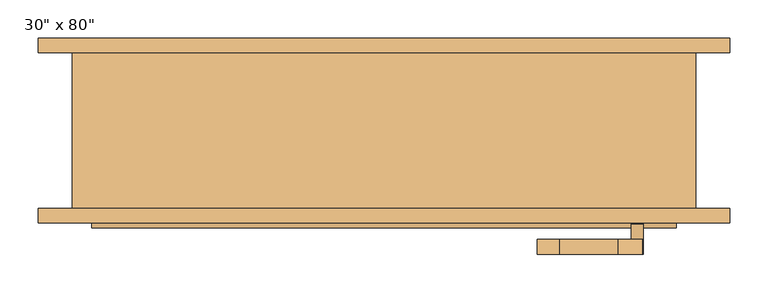
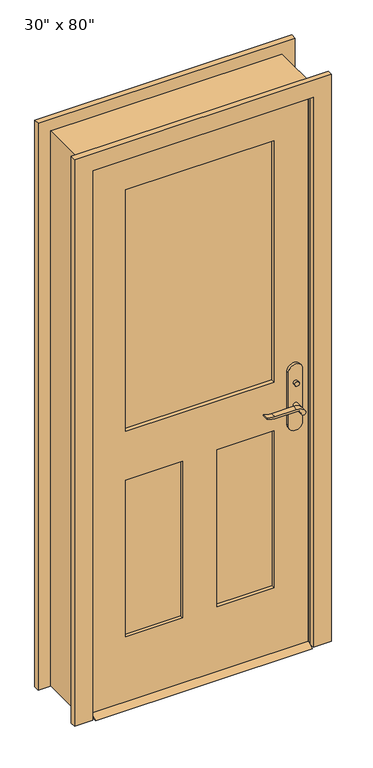
"""IFC4 building model written with IfcOpenShell, lengths in millimetres: door geometry."""

from ifc_helpers import new_model, si_unit, point, frame, frame_2d, origin, place, context, project, spatial, polyline, circle_curve, trimmed, segment, composite_curve, outline, extrude, faceted_brep, source, transform, mapped, element, save


def door_7e6851c9(model_context):
    return source(origin(), model_context, "Body", "SolidModel", [
        extrude(outline(polyline([(-63.5, 12.7), (-38.1, 0.0), (-123.825, 0.0), (-98.425, 12.7), (-63.5, 12.7)])), frame((-381.0, 0.0, 0.0), z_axis=(1.0, 0.0, 0.0), x_axis=(0.0, 1.0, 0.0)), (0.0, 0.0, 1.0), 762.0),
        extrude(outline(polyline([(335.2, -43.5), (335.2, -53.5), (325.2, -53.5), (325.2, -43.5), (335.2, -43.5)])), frame((0.0, 0.0, 981.9), z_axis=(0.0, 0.0, 1.0), x_axis=(1.0, 0.0, 0.0)), (0.0, 0.0, 1.0), 30.0),
        extrude(outline(composite_curve([segment(trimmed(circle_curve(frame_2d((996.9, 330.2)), 8.0), [point((996.9, 322.2))], [point((996.9, 338.2))], False, "CARTESIAN"), True, "CONTINUOUS"), segment(trimmed(circle_curve(frame_2d((996.9, 330.2)), 8.0), [point((996.9, 338.2))], [point((996.9, 322.2))], False, "CARTESIAN"), True, "CONTINUOUS")], self_intersect=False)), frame((0.0, -118.425, 0.0), z_axis=(0.0, 1.0, 0.0), x_axis=(0.0, 0.0, 1.0)), (0.0, 0.0, 1.0), 10.0),
        extrude(outline(composite_curve([segment(trimmed(circle_curve(frame_2d((897.1555521, 306.5324871)), 37.2832219), [point((919.0523287, 336.7081363))], [point((934.4, 304.8325667))], False, "CARTESIAN"), True, "CONTINUOUS"), segment(polyline([(934.4, 304.8325667), (934.4, 228.5564091)]), True, "CONTINUOUS"), segment(trimmed(circle_curve(frame_2d((1017.6850638, 228.6227909)), 83.2850902), [point((934.4, 228.5564091))], [point((939.4, 200.2))], True, "CARTESIAN"), True, "CONTINUOUS"), segment(polyline([(939.4, 200.2), (936.6135558, 200.2)]), True, "CONTINUOUS"), segment(trimmed(circle_curve(frame_2d((986.6709207, 232.1396612)), 59.3791355), [point((936.6135558, 200.2))], [point((927.4, 228.5564091))], False, "CARTESIAN"), True, "CONTINUOUS"), segment(polyline([(927.4, 228.5564091), (927.4, 304.8138099)]), True, "CONTINUOUS"), segment(trimmed(circle_curve(frame_2d((909.2738613, 304.8138099)), 18.1261387), [point((927.4, 304.8138099))], [point((914.4, 322.2))], True, "CARTESIAN"), True, "CONTINUOUS"), segment(trimmed(circle_curve(frame_2d((914.4, 330.2)), 8.0), [point((914.4, 322.2))], [point((919.0523287, 336.7081363))], False, "CARTESIAN"), True, "CONTINUOUS")], self_intersect=False)), frame((0.0, -23.5, 0.0), z_axis=(0.0, 1.0, 0.0), x_axis=(0.0, 0.0, 1.0)), (0.0, 0.0, 1.0), 20.0),
        extrude(outline(composite_curve([segment(trimmed(circle_curve(frame_2d((914.4, 330.2)), 8.0), [point((914.3999903, 322.2))], [point((919.0523287, 336.7081363))], False, "CARTESIAN"), True, "CONTINUOUS"), segment(trimmed(circle_curve(frame_2d((897.1555521, 306.5324871)), 37.2832219), [point((919.0523287, 336.7081363))], [point((934.4, 304.8325667))], False, "CARTESIAN"), True, "CONTINUOUS"), segment(polyline([(934.4, 304.8325667), (934.4, 228.5564091)]), True, "CONTINUOUS"), segment(trimmed(circle_curve(frame_2d((1017.6850638, 228.6227909)), 83.2850902), [point((934.4, 228.5564091))], [point((939.4, 200.2))], True, "CARTESIAN"), True, "CONTINUOUS"), segment(polyline([(939.4, 200.2), (936.6135558, 200.2)]), True, "CONTINUOUS"), segment(trimmed(circle_curve(frame_2d((986.6709207, 232.1396612)), 59.3791355), [point((936.6135558, 200.2))], [point((927.4, 228.5564091))], False, "CARTESIAN"), True, "CONTINUOUS"), segment(polyline([(927.4, 228.5564091), (927.4, 304.8138122)]), True, "CONTINUOUS"), segment(trimmed(circle_curve(frame_2d((909.2738682, 304.8138122)), 18.1261318), [point((927.4, 304.8138122))], [point((914.3999903, 322.2))], True, "CARTESIAN"), True, "CONTINUOUS")], self_intersect=False)), frame((0.0, -158.425, 0.0), z_axis=(0.0, 1.0, 0.0), x_axis=(0.0, 0.0, 1.0)), (0.0, 0.0, 1.0), 20.0),
        extrude(outline(composite_curve([segment(trimmed(circle_curve(frame_2d((914.4, 330.2)), 8.0), [point((914.4, 322.2))], [point((914.4, 338.2))], False, "CARTESIAN"), True, "CONTINUOUS"), segment(trimmed(circle_curve(frame_2d((914.4, 330.2)), 8.0), [point((914.4, 338.2))], [point((914.4, 322.2))], False, "CARTESIAN"), True, "CONTINUOUS")], self_intersect=False)), frame((0.0, -53.5, 0.0), z_axis=(0.0, 1.0, 0.0), x_axis=(0.0, 0.0, 1.0)), (0.0, 0.0, 1.0), 30.0),
        extrude(outline(composite_curve([segment(trimmed(circle_curve(frame_2d((914.4, 330.2)), 8.0), [point((914.4, 322.2))], [point((914.4, 338.2))], False, "CARTESIAN"), True, "CONTINUOUS"), segment(trimmed(circle_curve(frame_2d((914.4, 330.2)), 8.0), [point((914.4, 338.2))], [point((914.4, 322.2))], False, "CARTESIAN"), True, "CONTINUOUS")], self_intersect=False)), frame((0.0, -138.425, 0.0), z_axis=(0.0, 1.0, 0.0), x_axis=(0.0, 0.0, 1.0)), (0.0, 0.0, 1.0), 30.0),
        extrude(outline(composite_curve([segment(polyline([(844.4, 355.2), (1039.4, 355.2)]), True, "CONTINUOUS"), segment(trimmed(circle_curve(frame_2d((1039.4, 330.2)), 25.0), [point((1039.4, 355.2))], [point((1039.4, 305.2))], False, "CARTESIAN"), True, "CONTINUOUS"), segment(polyline([(1039.4, 305.2), (844.4, 305.2)]), True, "CONTINUOUS"), segment(trimmed(circle_curve(frame_2d((844.4, 330.2)), 25.0), [point((844.4, 305.2))], [point((844.4, 355.2))], False, "CARTESIAN"), True, "CONTINUOUS")], self_intersect=False)), frame((0.0, -63.5, 0.0), z_axis=(0.0, 1.0, 0.0), x_axis=(0.0, 0.0, 1.0)), (0.0, 0.0, 1.0), 10.0),
        extrude(outline(composite_curve([segment(polyline([(844.4, 355.2), (1039.4, 355.2)]), True, "CONTINUOUS"), segment(trimmed(circle_curve(frame_2d((1039.4, 330.2)), 25.0), [point((1039.4, 355.2))], [point((1039.4, 305.2))], False, "CARTESIAN"), True, "CONTINUOUS"), segment(polyline([(1039.4, 305.2), (844.4, 305.2)]), True, "CONTINUOUS"), segment(trimmed(circle_curve(frame_2d((844.4, 330.2)), 25.0), [point((844.4, 305.2))], [point((844.4, 355.2))], False, "CARTESIAN"), True, "CONTINUOUS")], self_intersect=False)), frame((0.0, -108.425, 0.0), z_axis=(0.0, 1.0, 0.0), x_axis=(0.0, 0.0, 1.0)), (0.0, 0.0, 1.0), 10.0),
        extrude(outline(polyline([(2032.0, -381.0), (12.7, -381.0), (12.7, 381.0), (2032.0, 381.0), (2032.0, -381.0)]), holes=[polyline([(1016.0, -260.35), (1911.35, -260.35), (1911.35, 260.35), (1016.0, 260.35), (1016.0, -260.35)]), polyline([(835.025, -60.325), (254.0, -60.325), (254.0, -260.35), (835.025, -260.35), (835.025, -60.325)]), polyline([(835.025, 260.35), (254.0, 260.35), (254.0, 60.325), (835.025, 60.325), (835.025, 260.35)])]), frame((0.0, -98.425, 0.0), z_axis=(0.0, 1.0, 0.0), x_axis=(0.0, 0.0, 1.0)), (0.0, 0.0, 1.0), 34.925),
        faceted_brep([(406.4, -98.425, 0.0), (381.0, -98.425, 0.0), (381.0, -63.5, 0.0), (368.3, -63.5, 0.0), (368.3, -28.575, 0.0), (381.0, -28.575, 0.0), (381.0, 104.775, 0.0), (406.4, 104.775, 0.0), (406.4, 104.775, 2057.4), (406.4, -98.425, 2057.4), (381.0, 104.775, 2032.0), (-381.0, 104.775, 2032.0), (-381.0, 104.775, 0.0), (-406.4, 104.775, 0.0), (-406.4, 104.775, 2057.4), (381.0, -28.575, 2032.0), (368.3, -28.575, 2019.3), (-368.3, -28.575, 2019.3), (-368.3, -28.575, 0.0), (-381.0, -28.575, 0.0), (-381.0, -28.575, 2032.0), (368.3, -63.5, 2019.3), (381.0, -63.5, 2032.0), (-381.0, -63.5, 2032.0), (-381.0, -63.5, 0.0), (-368.3, -63.5, 0.0), (-368.3, -63.5, 2019.3), (381.0, -98.425, 2032.0), (-406.4, -98.425, 2057.4), (-406.4, -98.425, 0.0), (-381.0, -98.425, 0.0), (-381.0, -98.425, 2032.0)], [[[0, 1, 2, 3, 4, 5, 6, 7]], [[7, 8, 9, 0]], [[6, 10, 11, 12, 13, 14, 8, 7]], [[5, 15, 10, 6]], [[4, 16, 17, 18, 19, 20, 15, 5]], [[3, 21, 16, 4]], [[2, 22, 23, 24, 25, 26, 21, 3]], [[1, 27, 22, 2]], [[0, 9, 28, 29, 30, 31, 27, 1]], [[8, 14, 28, 9]], [[15, 20, 11, 10]], [[21, 26, 17, 16]], [[27, 31, 23, 22]], [[29, 13, 12, 19, 18, 25, 24, 30]], [[14, 13, 29, 28]], [[20, 19, 12, 11]], [[26, 25, 18, 17]], [[31, 30, 24, 23]]]),
        extrude(outline(polyline([(-60.325, -75.1416667), (-60.325, -86.7833333), (-260.35, -86.7833333), (-260.35, -75.1416667), (-60.325, -75.1416667)])), frame((0.0, 0.0, 254.0), z_axis=(0.0, 0.0, 1.0), x_axis=(1.0, 0.0, 0.0)), (0.0, 0.0, 1.0), 581.025),
        extrude(outline(polyline([(260.35, -75.1416667), (260.35, -86.7833333), (60.325, -86.7833333), (60.325, -75.1416667), (260.35, -75.1416667)])), frame((0.0, 0.0, 254.0), z_axis=(0.0, 0.0, 1.0), x_axis=(1.0, 0.0, 0.0)), (0.0, 0.0, 1.0), 581.025),
        extrude(outline(polyline([(260.35, -77.47), (260.35, -84.455), (-260.35, -84.455), (-260.35, -77.47), (260.35, -77.47)])), frame((0.0, 0.0, 1016.0), z_axis=(0.0, 0.0, 1.0), x_axis=(1.0, 0.0, 0.0)), (0.0, 0.0, 1.0), 895.35),
        extrude(outline(polyline([(0.0, -387.35), (2038.35, -387.35), (2038.35, 387.35), (0.0, 387.35), (0.0, 450.85), (2101.85, 450.85), (2101.85, -450.85), (0.0, -450.85), (0.0, -387.35)])), frame((0.0, 104.775, 0.0), z_axis=(0.0, 1.0, 0.0), x_axis=(0.0, 0.0, 1.0)), (0.0, 0.0, 1.0), 19.05),
        extrude(outline(polyline([(0.0, -387.35), (2038.35, -387.35), (2038.35, 387.35), (0.0, 387.35), (0.0, 450.85), (2101.85, 450.85), (2101.85, -450.85), (0.0, -450.85), (0.0, -387.35)])), frame((0.0, -117.475, 0.0), z_axis=(0.0, 1.0, 0.0), x_axis=(0.0, 0.0, 1.0)), (0.0, 0.0, 1.0), 19.05),
    ])


if __name__ == "__main__":
    model = new_model("IFC4")
    model_context = context("Model", 3, world=origin())
    ifc_project = project(units=[si_unit("LENGTHUNIT", "METRE", prefix="MILLI")], contexts=[model_context])
    site = spatial("IfcSite", under=ifc_project)
    building = spatial("IfcBuilding", under=site)
    placement = place(None, origin())
    door_shape = door_7e6851c9(model_context)
    element("IfcDoor", 1, ObjectType="30\" x 80\"", at=placement, inside=building, context=model_context, shape_type="MappedRepresentation", body=[
        mapped(door_shape, transform((0.0, 0.0, 0.0), x_axis=(1.0, 0.0, 0.0), y_axis=(0.0, 1.0, 0.0), z_axis=(0.0, 0.0, 1.0))),
    ])
    save(model, "model.ifc")

# Revit data of these elements
# Type "30\" x 80\""
#   Type Mark = "10"
#   Assembly Code = "B2030100"
#   Analytic Construction = "French door, wood frame with single glass"
#   Top Rail = 0' - 4 3/4"
#   Threshold Offset [instance default] = 0' - 0 1/2"
#   Thickness = 0' - 1 3/8"
#   Thermal Resistance (R) = 1.0696 (h·ft²·°F)/BTU
#   Swing Angle [instance default] = 90.00°
#   Stiles = 0' - 4 3/4"
#   Rough Width = 2' - 8"
#   Rough Height = 6' - 9"
#   Lock Rail = 0' - 7 1/8"
#   Height = 6' - 8"
#   Width = 2' - 6"
#   Heat Transfer Coefficient (U) = 0.9350 BTU/(h·ft²·°F)
#   Door Offset [instance default] = 0' - 0"
#   Bottom Rail = 0' - 9 1/2"
#   Threshold [instance default] = yes
#   Function = 1
#   Exterior Trim [instance default] = yes
#   Trim Material = Cherry
#   Threshold Material = Cherry
#   Panel Material = Cherry
#   Glazing = Glass
#   Frame Material = Cherry
#   Door Handle Material = Aluminum
#   Visual Light Transmittance = 0
#   Solar Heat Gain Coefficient = 0
#   Wall Closure = (empty or 0)
#   Construction Type = (empty or 0)
# Element 1 (IfcDoor, "30\" x 80\"")
#   Materials on its faces: "Cherry", "Aluminum", "Glass"
# Materials
#   "Cherry": class "Wood", colour RGB 226 177 128, transparency 0, Description = "Prunus Serotina", Cost = 0
#   "Glass": class "Glass", colour RGB 0 128 192, transparency 0.75, Description = "Soda Lime Glass", Cost = 0
#   "Aluminum": class "Metal", colour RGB 247 247 247, transparency 0, Description = "Aluminum 6061", Cost = 0
